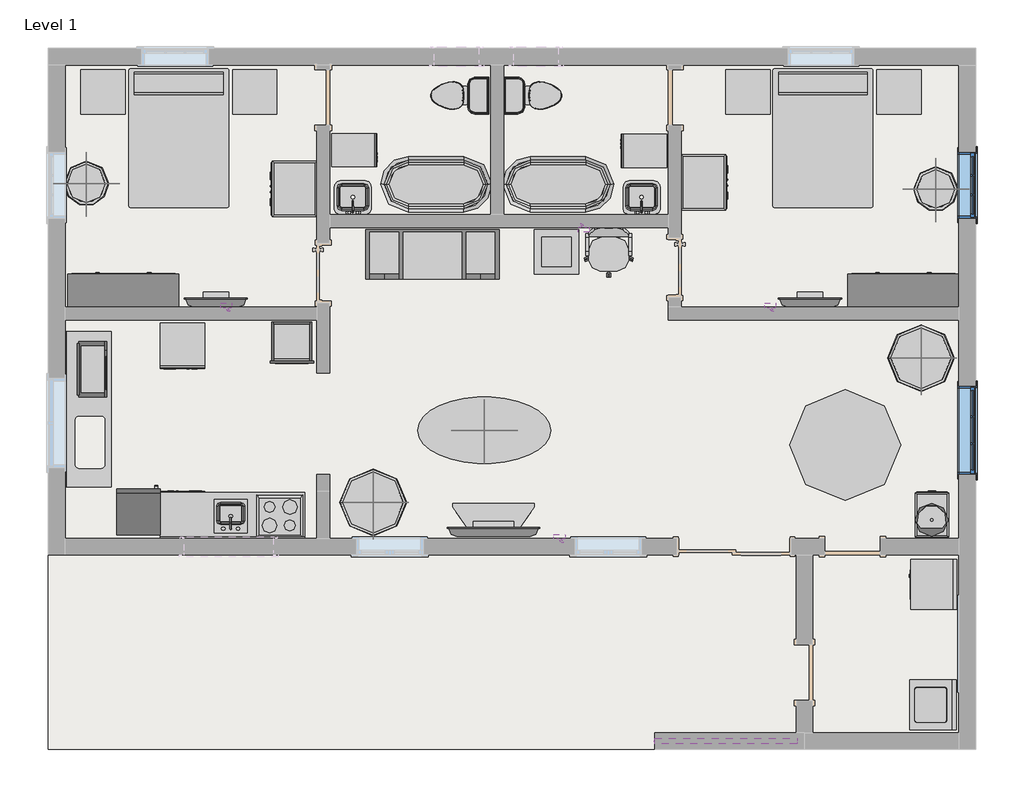
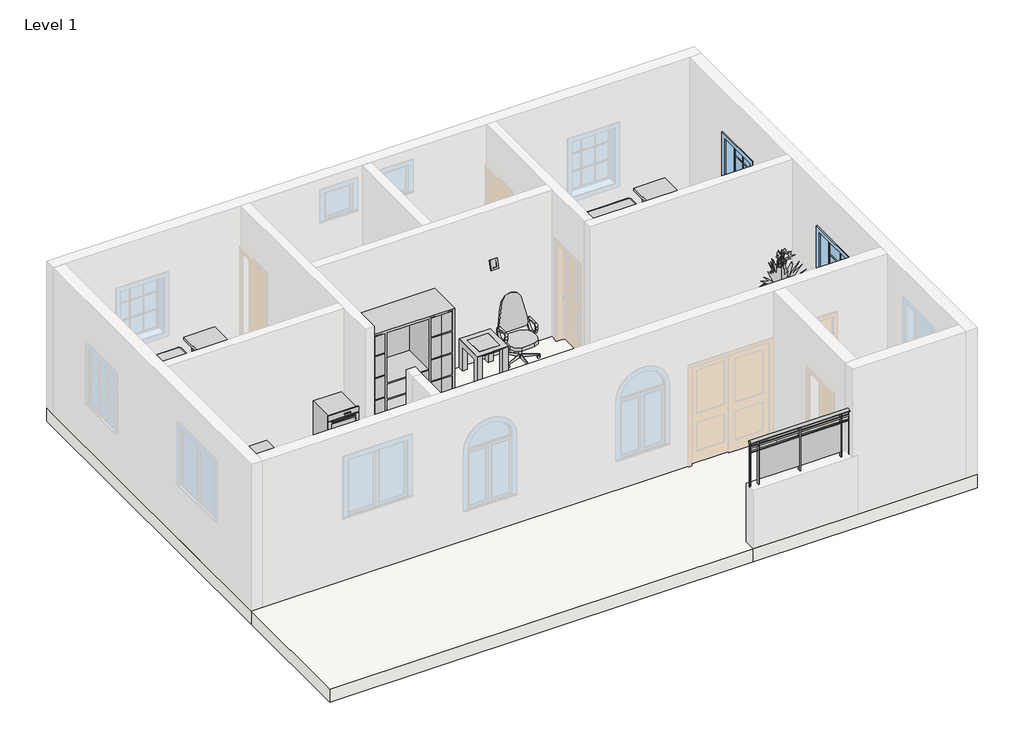
# One storey, part 2 of 2: 26 furniture elements, 15 proxies, 11 flow terminals, 5 geographic elements, 2 windows, 1 railing, 1 slab.
# Revit data of these elements (continued)
# Materials (continued)
#   "Cabinets - Handles": class "Metal", colour RGB 57 57 57, transparency 0
#   "Laminate, Ivory, Matte": class "Plastic", colour RGB 247 247 239, transparency 0, Description = "Plastic Laminate - Ivory, Matte", Cost = 0
#   "Metal - Stainless Steel, Polished": class "Metal", colour RGB 216 216 216, transparency 0
#   "Porcelain, Linen": class "Ceramic", colour RGB 249 239 230, transparency 0, Description = "Porcelain, linen", Cost = 0
#   "Laminate, Linen, Matte": class "Plastic", colour RGB 249 239 230, transparency 0, Description = "Plastic Laminate - Linen, Matte", Cost = 0
#   "Porcelain, Ivory": class "Ceramic", colour RGB 247 247 239, transparency 0, Description = "Porcelain, ivory", Cost = 0
#   "Plywood, Sheathing": class "Wood", colour RGB 212 179 113, transparency 0, Description = "Plywood, sheathing grade", Cost = 0
#   "Textile - Slate Blue": class "Fabric", colour RGB 98 102 118, transparency 0
#   "Laminate - Ivory, Glossy": colour RGB 247 247 239, transparency 0
#   "Cherry": class "Wood", colour RGB 226 177 128, transparency 0, Description = "Prunus Serotina", Cost = 0
#   "Wood - Teak": class "Wood", colour RGB 145 112 90, transparency 0
#   "Melamine - Gray": class "Wood", colour RGB 49 49 49, transparency 0
#   "Pine": class "Wood", colour RGB 223 192 134, transparency 0, Description = "Pinus Echinata", Cost = 0
#   "Birch": class "Wood", colour RGB 224 178 126, transparency 0, Description = "Betula Alleghaniensis", Cost = 0
#   "Laminate - Black": colour RGB 0 0 0, transparency 0
#   "Tile, Mosaic, Gray": class "Generic", colour RGB 127 127 127, transparency 0, Description = "Mosiac tile, gray", Cost = 0
#   "Concrete, Cast-in-Place gray": class "Concrete", colour RGB 192 192 192, transparency 0, Description = "Cast-in-place concrete", Cost = 0
#   "Structure, Wood Joist/Rafter Layer": class "Wood", colour RGB 127 127 127, transparency 0, Description = "Wood framing, thermal airspace", Cost = 0
#   "Glass": class "Glass", colour RGB 0 128 192, transparency 0.75, Description = "Soda Lime Glass", Cost = 0
#   "Softwood, Lumber": class "Wood", colour RGB 223 192 134, transparency 0, Description = "Pinus Echinata", Cost = 0
#   "Trim": class "Wood", colour RGB 224 178 126, transparency 0
#   "Sash": class "Wood", colour RGB 224 178 126, transparency 0
#   "Steel": class "Metal", colour RGB 247 247 247, transparency 0, Description = "Steel, mill finish", Cost = 0
#   "Linen, White": class "Textile", colour RGB 247 247 239, transparency 0, Description = "Linen, white", Cost = 0
#   "Counter Top": class "Wood", colour RGB 226 177 128, transparency 0
#   "Glass - Clear, Grey": class "Glass", colour RGB 252 255 255, transparency 0.64
#   "TV - Black": colour RGB 49 49 49, transparency 0
#   "TV - Glass": colour RGB 157 157 157, transparency 0.9
#   "TV - Screen": colour RGB 0 0 0, transparency 0
#   "Glass - Shelves": class "Glass", colour RGB 167 167 167, transparency 0.9
